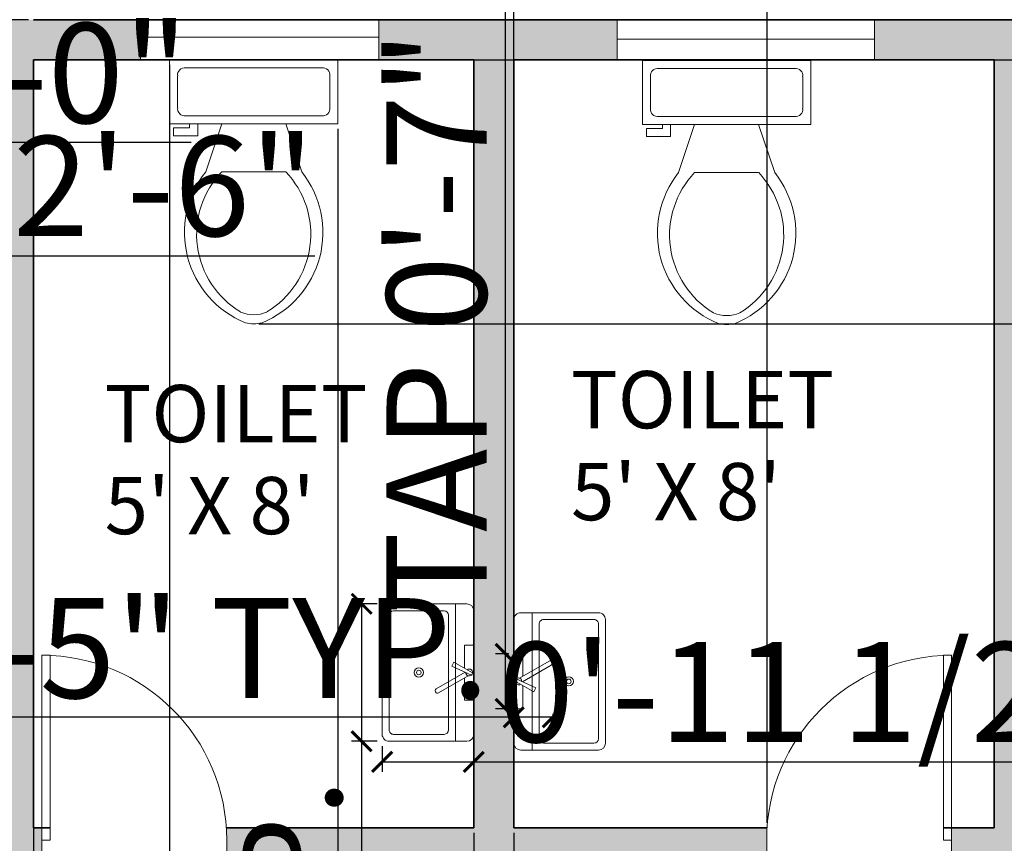
# Model space of a CAD drawing. Units: inches. Extents: x 1763 to 2368, y 1500 to 2097.
# Tile 11 of 24: x 1956 to 2079, y 1883 to 1986. Entities that reach past the tile are written whole.
import ezdxf

# ---------------------------------------------------------------- set-up
doc = ezdxf.new("R2010")
doc.units = ezdxf.units.IN
for name, color, linetype, lineweight in [('A-ANNO-DIMS', 2, 'Continuous', 18), ('A-AREA-IDEN', 7, 'Continuous', 18), ('A-DOOR', 4, 'Continuous', 18), ('A-FLOR-FIXT', 9, 'Continuous', 18), ('A-WALL', 7, 'Continuous', 35), ('A-WALL-PATT', 7, 'Continuous', 13), ('windows', 1, 'Continuous', 18)]:
    doc.layers.add(name, color=color, linetype=linetype, lineweight=lineweight)
doc.styles.get("Standard").update_dxf_attribs({"font": 'arial.ttf'})
doc.dimstyles.new('ISO-25', dxfattribs={"dimtxt": 12.5, "dimasz": 2.5, "dimexe": 1.25, "dimexo": 0.625, "dimtad": 1, "dimdec": 0, "dimlunit": 4, "dimtxsty": 'Standard', "dimblk": 'ARCHTICK', "dimcen": 2.5, "dimclrd": 3, "dimclrt": 4, "dimadec": 0, "dimazin": 0, "dimtfac": 1, "dimtdec": 0, "dimtmove": 0, "dimatfit": 3, "dimfxl": 1, "dimarcsym": 0})

# ---------------------------------------------------------------- blocks, each defined once
blk = doc.blocks.new('*U3')
for p, q in [((0, 0), (0, -6)), ((40, 0), (40, -6))]:
    blk.add_line(p, q)
blk.add_lwpolyline([(0, 0), (0, 40), (1.75, 40), (1.75, 0)], close=True)
blk.add_arc((0, 0), 40, 0, 90)
blk = doc.blocks.new('*U5')
for p, q in [((9.5, -6), (9.5, -2)), ((-10, -8.5), (-8, -8.5)), ((-10, -9.5), (-10, -8.5)), ((-8, -8.5), (-8, -8)), ((-7, -8), (-7, -9.5)), ((-4, -8), (-6, -14)), ((4, -8), (6, -14)), ((-7, -9.5), (-10, -9.5)), ((4, -14), (-4, -14))]:
    blk.add_line(p, q)
blk.add_lwpolyline([(10.5, -8), (10.5, 0), (-10.5, 0), (-10.5, -8)], close=True)
for points in [[(8.5, -1), (-8.5, -1)], [(-9.5, -2), (-9.5, -6)], [(-8.5, -7), (8.5, -7)]]:
    blk.add_lwpolyline(points)
for centre, radius, start, end in [((-8.62, -1.88), 0.884, 81.8699, 188.1301), ((8.62, -1.88), 0.884, 351.8699, 98.1301), ((-8.62, -6.12), 0.884, 171.8699, 278.1301), ((8.62, -6.12), 0.884, 261.8699, 8.1301), ((3.52, -21.58), 12.17, 141.4691, 247.9714), ((4.2, -21.82), 11.33, 136.3677, 238.9468), ((-3.52, -21.58), 12.17, 292.0284, 38.5307), ((-4.2, -21.82), 11.33, 301.053, 43.6321), ((0, -27.88), 4, 245.7318, 294.2682), ((0, -29), 4, 254.8605, 285.1395)]:
    blk.add_arc(centre, radius, start, end)
blk = doc.blocks.new('Faucet - single handle top')
for p, q in [((0.08, -0.26), (-2.26, -4.34)), ((-1.37, -4.79), (0.55, -0.5)), ((-0.06, -1.9), (3.57, -8.18)), ((4.43, -7.68), (0.72, -1.24)), ((-2.26, -4.34), (-1.37, -4.79))]:
    blk.add_line(p, q)
for points in [[(-0.92, -2), (-6, -2), (-6, 0), (6, 0), (6, -2), (1.16, -2)], [(-0.01, -2), (-0.12, -2)]]:
    blk.add_lwpolyline(points)
for centre, radius, start, end in [((0, -1), 0.75, 269.2246, 216.2304), ((4, -7.93), 0.5, 210, 30)]:
    blk.add_arc(centre, radius, start, end)
blk = doc.blocks.new('Sink-single - 30 in top')
blk.add_line((-15, -3.999996), (15, -3.999996))
for points in [[(-13.5, 0), (13.5, 0)], [(-15, -18.499996), (-15, -1.5)], [(15, -1.5), (15, -18.499996)], [(-12.5, -5.499996), (12.5, -5.499996)], [(-13.5, -17.499996), (-13.5, -6.499996)], [(13.5, -6.499996), (13.5, -17.499996)], [(12.5, -18.499996), (-12.5, -18.499996)], [(13.5, -19.999996), (-13.5, -19.999996)]]:
    blk.add_lwpolyline(points)
for radius in [1, 0.5]:
    blk.add_circle((0, -11.999996), radius)
for centre, radius, start, end in [((-13.5, -1.5), 1.5, 90, 180), ((13.5, -1.5), 1.5, 0, 90), ((-12.5, -6.499996), 1, 90, 180), ((12.5, -6.499996), 1, 0, 90), ((-13.5, -18.499996), 1.5, 180, 270), ((-12.5, -17.499996), 1, 180, 270), ((12.5, -17.499996), 1, 270, 0), ((13.5, -18.499996), 1.5, 270, 0)]:
    blk.add_arc(centre, radius, start, end)
blk = doc.blocks.new('_ArchTick')
at = {"color": 0, "linetype": 'ByBlock', "const_width": 0.15}
blk.add_lwpolyline([(-0.5, -0.5), (0.5, 0.5)], dxfattribs=at)
blk = doc.blocks.new('*D31')
at = {"layer": 'A-ANNO-DIMS', "color": 0, "lineweight": -2, "transparency": 16777216}
for p, q in [((1880.68, 1960.65), (1880.68, 1955.52)), ((1910.68, 1960.65), (1910.68, 1955.52))]:
    blk.add_line(p, q, dxfattribs=at)
at = {"layer": 'A-ANNO-DIMS', "color": 3, "lineweight": -2, "transparency": 16777216}
for p, q in [((1880.68, 1956.77), (1910.68, 1956.77)), ((1910.68, 1956.77), (1993.21, 1956.77))]:
    blk.add_line(p, q, dxfattribs=at)
at = {"layer": 'Defpoints', "color": 0, "transparency": 16777216}
for p in [(1880.68, 1961.27), (1910.68, 1961.27), (1910.68, 1956.77)]:
    blk.add_point(p, dxfattribs=at)
at = {"layer": 'A-ANNO-DIMS', "color": 3, "lineweight": -2, "transparency": 16777216, "xscale": 2.5, "yscale": 2.5, "zscale": 2.5, "rotation": 180}
blk.add_blockref('_ArchTick', (1880.68, 1956.77), dxfattribs=at)
at = {"layer": 'A-ANNO-DIMS', "color": 3, "lineweight": -2, "transparency": 16777216, "xscale": 2.5, "yscale": 2.5, "zscale": 2.5}
blk.add_blockref('_ArchTick', (1910.68, 1956.77), dxfattribs=at)
at = {"layer": 'A-ANNO-DIMS', "color": 4, "transparency": 16777216, "insert": (1953.2, 1963.86), "char_height": 12.5, "attachment_point": 5}
blk.add_mtext('SINK 2\'-6"', dxfattribs=at)
blk = doc.blocks.new('*D33')
at = {"layer": 'A-ANNO-DIMS', "color": 0, "lineweight": -2, "transparency": 16777216}
for p, q in [((2001.02, 1913.28), (1997.82, 1913.28)), ((2001.02, 1896.11), (1997.82, 1896.11))]:
    blk.add_line(p, q, dxfattribs=at)
at = {"layer": 'A-ANNO-DIMS', "color": 3, "lineweight": -2, "transparency": 16777216}
for p, q in [((1999.07, 1913.28), (1999.07, 1896.11)), ((1999.07, 1896.11), (1999.07, 1770.61))]:
    blk.add_line(p, q, dxfattribs=at)
at = {"layer": 'Defpoints', "color": 0, "transparency": 16777216}
for p in [(2001.64, 1913.28), (1999.07, 1896.11), (2001.64, 1896.11)]:
    blk.add_point(p, dxfattribs=at)
at = {"layer": 'A-ANNO-DIMS', "color": 3, "lineweight": -2, "transparency": 16777216, "xscale": 2.5, "yscale": 2.5, "zscale": 2.5}
for p, rotation in [((1999.07, 1913.28), 90), ((1999.07, 1896.11), 270)]:
    blk.add_blockref('_ArchTick', p, dxfattribs=dict(at, rotation=rotation))
at = {"layer": 'A-ANNO-DIMS', "color": 4, "transparency": 16777216, "insert": (1991.98, 1832.11), "char_height": 12.5, "attachment_point": 5, "rotation": 90}
blk.add_mtext('SINK 1\'-5" TYP.', dxfattribs=at)
blk = doc.blocks.new('*D34')
at = {"layer": 'A-ANNO-DIMS', "color": 0, "lineweight": -2, "transparency": 16777216}
for p, q in [((2001.64, 1895.48), (2001.64, 1892.28)), ((2013.09, 1895.48), (2013.09, 1892.28))]:
    blk.add_line(p, q, dxfattribs=at)
at = {"layer": 'A-ANNO-DIMS', "color": 3, "lineweight": -2, "transparency": 16777216}
for p, q in [((2001.64, 1893.53), (2013.09, 1893.53)), ((2013.09, 1893.53), (2131.87, 1893.53))]:
    blk.add_line(p, q, dxfattribs=at)
at = {"layer": 'Defpoints', "color": 0, "transparency": 16777216}
for p in [(2001.64, 1896.11), (2013.09, 1896.11), (2013.09, 1893.53)]:
    blk.add_point(p, dxfattribs=at)
at = {"layer": 'A-ANNO-DIMS', "color": 3, "lineweight": -2, "transparency": 16777216, "xscale": 2.5, "yscale": 2.5, "zscale": 2.5, "rotation": 180}
blk.add_blockref('_ArchTick', (2001.64, 1893.53), dxfattribs=at)
at = {"layer": 'A-ANNO-DIMS', "color": 3, "lineweight": -2, "transparency": 16777216, "xscale": 2.5, "yscale": 2.5, "zscale": 2.5}
blk.add_blockref('_ArchTick', (2013.09, 1893.53), dxfattribs=at)
at = {"layer": 'A-ANNO-DIMS', "color": 4, "transparency": 16777216, "insert": (2073.73, 1900.62), "char_height": 12.5, "attachment_point": 5}
blk.add_mtext('0\'-11 1/2" TYP.', dxfattribs=at)
blk = doc.blocks.new('*D35')
at = {"layer": 'A-ANNO-DIMS', "color": 0, "lineweight": -2, "transparency": 16777216}
for p, q in [((1889.68, 1972.15), (1889.68, 1969.72)), ((1901.68, 1972.15), (1901.68, 1969.72))]:
    blk.add_line(p, q, dxfattribs=at)
at = {"layer": 'A-ANNO-DIMS', "color": 3, "lineweight": -2, "transparency": 16777216}
for p, q in [((1889.68, 1970.97), (1901.68, 1970.97)), ((1901.68, 1970.97), (1977.79, 1970.97))]:
    blk.add_line(p, q, dxfattribs=at)
at = {"layer": 'Defpoints', "color": 0, "transparency": 16777216}
for p in [(1889.68, 1972.77), (1901.68, 1972.77), (1901.68, 1970.97)]:
    blk.add_point(p, dxfattribs=at)
at = {"layer": 'A-ANNO-DIMS', "color": 3, "lineweight": -2, "transparency": 16777216, "xscale": 2.5, "yscale": 2.5, "zscale": 2.5, "rotation": 180}
blk.add_blockref('_ArchTick', (1889.68, 1970.97), dxfattribs=at)
at = {"layer": 'A-ANNO-DIMS', "color": 3, "lineweight": -2, "transparency": 16777216, "xscale": 2.5, "yscale": 2.5, "zscale": 2.5}
blk.add_blockref('_ArchTick', (1901.68, 1970.97), dxfattribs=at)
at = {"layer": 'A-ANNO-DIMS', "color": 4, "transparency": 16777216, "insert": (1940.99, 1977.98), "char_height": 12.5, "attachment_point": 5}
blk.add_mtext('TAP 1\'-0"', dxfattribs=at)
blk = doc.blocks.new('*D37')
at = {"layer": 'A-ANNO-DIMS', "color": 3, "lineweight": -2, "transparency": 16777216}
for p, q in [((2017.06, 1907.01), (2017.06, 2026.09)), ((2017.06, 1900.14), (2017.06, 1907.01))]:
    blk.add_line(p, q, dxfattribs=at)
at = {"layer": 'A-ANNO-DIMS', "color": 0, "lineweight": -2, "transparency": 16777216}
for p, q in [((2017.47, 1907.01), (2015.81, 1907.01)), ((2017.47, 1900.14), (2015.81, 1900.14))]:
    blk.add_line(p, q, dxfattribs=at)
at = {"layer": 'Defpoints', "color": 0, "transparency": 16777216}
for p in [(2017.06, 1907.01), (2018.09, 1907.01), (2018.09, 1900.14)]:
    blk.add_point(p, dxfattribs=at)
at = {"layer": 'A-ANNO-DIMS', "color": 3, "lineweight": -2, "transparency": 16777216, "xscale": 2.5, "yscale": 2.5, "zscale": 2.5}
for p, rotation in [((2017.06, 1907.01), 90), ((2017.06, 1900.14), 270)]:
    blk.add_blockref('_ArchTick', p, dxfattribs=dict(at, rotation=rotation))
at = {"layer": 'A-ANNO-DIMS', "color": 4, "transparency": 16777216, "insert": (2010.05, 1967.8), "char_height": 12.5, "attachment_point": 5, "rotation": 90}
blk.add_mtext('TAP 0\'-7" TYP.', dxfattribs=at)
blk = doc.blocks.new('*D38')
at = {"layer": 'A-ANNO-DIMS', "color": 0, "lineweight": -2, "transparency": 16777216}
for p, q in [((2018.09, 1899.52), (2018.09, 1897.86)), ((2022.96, 1899.52), (2022.96, 1897.86))]:
    blk.add_line(p, q, dxfattribs=at)
at = {"layer": 'A-ANNO-DIMS', "color": 3, "lineweight": -2, "transparency": 16777216}
for p, q in [((2018.09, 1899.11), (1938.15, 1899.11)), ((2022.96, 1899.11), (2018.09, 1899.11))]:
    blk.add_line(p, q, dxfattribs=at)
at = {"layer": 'Defpoints', "color": 0, "transparency": 16777216}
for p in [(2018.09, 1900.14), (2022.96, 1900.14), (2018.09, 1899.11)]:
    blk.add_point(p, dxfattribs=at)
at = {"layer": 'A-ANNO-DIMS', "color": 3, "lineweight": -2, "transparency": 16777216, "xscale": 2.5, "yscale": 2.5, "zscale": 2.5, "rotation": 180}
blk.add_blockref('_ArchTick', (2018.09, 1899.11), dxfattribs=at)
at = {"layer": 'A-ANNO-DIMS', "color": 3, "lineweight": -2, "transparency": 16777216, "xscale": 2.5, "yscale": 2.5, "zscale": 2.5}
blk.add_blockref('_ArchTick', (2022.96, 1899.11), dxfattribs=at)
at = {"layer": 'A-ANNO-DIMS', "color": 4, "transparency": 16777216, "insert": (1976.87, 1906.12), "char_height": 12.5, "attachment_point": 5}
blk.add_mtext('0\'-5" TYP.', dxfattribs=at)
blk = doc.blocks.new('*D58')
at = {"layer": 'A-ANNO-DIMS', "color": 0, "lineweight": -2, "transparency": 16777216}
for p, q in [((1871.68, 1635.9), (1871.68, 2072.02)), ((1927.07, 1635.9), (1927.07, 2072.02))]:
    blk.add_line(p, q, dxfattribs=at)
at = {"layer": 'A-ANNO-DIMS', "color": 3, "lineweight": -2, "transparency": 16777216}
for p, q in [((1871.68, 2070.77), (1927.07, 2070.77)), ((1927.07, 2070.77), (1993.68, 2070.77))]:
    blk.add_line(p, q, dxfattribs=at)
at = {"layer": 'Defpoints', "color": 0, "transparency": 16777216}
for p in [(1927.07, 2070.77), (1871.68, 1635.27), (1927.07, 1635.27)]:
    blk.add_point(p, dxfattribs=at)
at = {"layer": 'A-ANNO-DIMS', "color": 3, "lineweight": -2, "transparency": 16777216, "xscale": 2.5, "yscale": 2.5, "zscale": 2.5, "rotation": 180}
blk.add_blockref('_ArchTick', (1871.68, 2070.77), dxfattribs=at)
at = {"layer": 'A-ANNO-DIMS', "color": 3, "lineweight": -2, "transparency": 16777216, "xscale": 2.5, "yscale": 2.5, "zscale": 2.5}
blk.add_blockref('_ArchTick', (1927.07, 2070.77), dxfattribs=at)
at = {"layer": 'A-ANNO-DIMS', "color": 4, "transparency": 16777216, "insert": (1961.63, 2077.86), "char_height": 12.5, "attachment_point": 5}
blk.add_mtext('4\'-7 1/2"', dxfattribs=at)
blk = doc.blocks.new('*D72')
at = {"layer": 'A-ANNO-DIMS', "color": 0, "lineweight": -2, "transparency": 16777216}
for p, q in [((2018.09, 1885.9), (2018.09, 2072.02)), ((2049.74, 1885.9), (2049.74, 2072.02))]:
    blk.add_line(p, q, dxfattribs=at)
at = {"layer": 'A-ANNO-DIMS', "color": 3, "lineweight": -2, "transparency": 16777216}
for p, q in [((2018.09, 2070.77), (2049.74, 2070.77)), ((2049.74, 2070.77), (2116.06, 2070.77))]:
    blk.add_line(p, q, dxfattribs=at)
at = {"layer": 'Defpoints', "color": 0, "transparency": 16777216}
for p in [(2049.74, 2070.77), (2018.09, 1885.27), (2049.74, 1885.27)]:
    blk.add_point(p, dxfattribs=at)
at = {"layer": 'A-ANNO-DIMS', "color": 3, "lineweight": -2, "transparency": 16777216, "xscale": 2.5, "yscale": 2.5, "zscale": 2.5, "rotation": 180}
blk.add_blockref('_ArchTick', (2018.09, 2070.77), dxfattribs=at)
at = {"layer": 'A-ANNO-DIMS', "color": 3, "lineweight": -2, "transparency": 16777216, "xscale": 2.5, "yscale": 2.5, "zscale": 2.5}
blk.add_blockref('_ArchTick', (2049.74, 2070.77), dxfattribs=at)
at = {"layer": 'A-ANNO-DIMS', "color": 4, "transparency": 16777216, "insert": (2084.15, 2077.86), "char_height": 12.5, "attachment_point": 5}
blk.add_mtext('2\'-7 1/2"', dxfattribs=at)
blk = doc.blocks.new('*D77')
at = {"layer": 'A-ANNO-DIMS', "color": 0, "lineweight": -2, "transparency": 16777216}
for p, q in [((1975.09, 1972.65), (1975.09, 1509.91)), ((1996.09, 1972.65), (1996.09, 1509.91))]:
    blk.add_line(p, q, dxfattribs=at)
at = {"layer": 'A-ANNO-DIMS', "color": 3, "lineweight": -2, "transparency": 16777216}
for p, q in [((1975.09, 1511.16), (1996.09, 1511.16)), ((1996.09, 1511.16), (2031.89, 1511.16))]:
    blk.add_line(p, q, dxfattribs=at)
at = {"layer": 'Defpoints', "color": 0, "transparency": 16777216}
for p in [(1975.09, 1973.27), (1996.09, 1973.27), (1996.09, 1511.16)]:
    blk.add_point(p, dxfattribs=at)
at = {"layer": 'A-ANNO-DIMS', "color": 3, "lineweight": -2, "transparency": 16777216, "xscale": 2.5, "yscale": 2.5, "zscale": 2.5, "rotation": 180}
blk.add_blockref('_ArchTick', (1975.09, 1511.16), dxfattribs=at)
at = {"layer": 'A-ANNO-DIMS', "color": 3, "lineweight": -2, "transparency": 16777216, "xscale": 2.5, "yscale": 2.5, "zscale": 2.5}
blk.add_blockref('_ArchTick', (1996.09, 1511.16), dxfattribs=at)
at = {"layer": 'A-ANNO-DIMS', "color": 4, "transparency": 16777216, "insert": (2015.24, 1518.16), "char_height": 12.5, "attachment_point": 5}
blk.add_mtext('1\'-9"', dxfattribs=at)
blk = doc.blocks.new('*D78')
at = {"layer": 'A-ANNO-DIMS', "color": 0, "lineweight": -2, "transparency": 16777216}
for p, q in [((1996.72, 1981.27), (2217.84, 1981.27)), ((1986.22, 1948.27), (2217.84, 1948.27))]:
    blk.add_line(p, q, dxfattribs=at)
at = {"layer": 'A-ANNO-DIMS', "color": 3, "lineweight": -2, "transparency": 16777216}
for p, q in [((2216.59, 1981.27), (2216.59, 1948.27)), ((2216.59, 1948.27), (2216.59, 1911.08))]:
    blk.add_line(p, q, dxfattribs=at)
at = {"layer": 'Defpoints', "color": 0, "transparency": 16777216}
for p in [(1996.09, 1981.27), (1985.59, 1948.27), (2216.59, 1948.27)]:
    blk.add_point(p, dxfattribs=at)
at = {"layer": 'A-ANNO-DIMS', "color": 3, "lineweight": -2, "transparency": 16777216, "xscale": 2.5, "yscale": 2.5, "zscale": 2.5}
for p, rotation in [((2216.59, 1981.27), 90), ((2216.59, 1948.27), 270)]:
    blk.add_blockref('_ArchTick', p, dxfattribs=dict(at, rotation=rotation))
at = {"layer": 'A-ANNO-DIMS', "color": 4, "transparency": 16777216, "insert": (2209.58, 1928.43), "char_height": 12.5, "attachment_point": 5, "rotation": 90}
blk.add_mtext('2\'-9"', dxfattribs=at)
blk = doc.blocks.new('*D81')
at = {"layer": 'A-ANNO-DIMS', "color": 3, "lineweight": -2, "transparency": 16777216}
for p, q in [((1788.85, 1866.87), (1788.85, 1912.38)), ((1788.85, 1843.77), (1788.85, 1866.87))]:
    blk.add_line(p, q, dxfattribs=at)
at = {"layer": 'A-ANNO-DIMS', "color": 0, "lineweight": -2, "transparency": 16777216}
for p, q in [((2077.47, 1866.87), (1787.6, 1866.87)), ((2077.47, 1843.77), (1787.6, 1843.77))]:
    blk.add_line(p, q, dxfattribs=at)
at = {"layer": 'Defpoints', "color": 0, "transparency": 16777216}
for p in [(1788.85, 1866.87), (2078.09, 1866.87), (2078.09, 1843.77)]:
    blk.add_point(p, dxfattribs=at)
at = {"layer": 'A-ANNO-DIMS', "color": 3, "lineweight": -2, "transparency": 16777216, "xscale": 2.5, "yscale": 2.5, "zscale": 2.5}
for p, rotation in [((1788.85, 1866.87), 90), ((1788.85, 1843.77), 270)]:
    blk.add_blockref('_ArchTick', p, dxfattribs=dict(at, rotation=rotation))
at = {"layer": 'A-ANNO-DIMS', "color": 4, "transparency": 16777216, "insert": (1781.95, 1890.87), "char_height": 12.5, "attachment_point": 5, "rotation": 90}
blk.add_mtext('1\'-11"', dxfattribs=at)
blk = doc.blocks.new('*D82')
at = {"layer": 'A-ANNO-DIMS', "color": 3, "lineweight": -2, "transparency": 16777216}
for p, q in [((1788.85, 1843.77), (1788.85, 1909.87)), ((1788.85, 1837.27), (1788.85, 1843.77))]:
    blk.add_line(p, q, dxfattribs=at)
at = {"layer": 'A-ANNO-DIMS', "color": 0, "lineweight": -2, "transparency": 16777216}
for p, q in [((2077.47, 1843.77), (1787.6, 1843.77)), ((2077.47, 1837.27), (1787.6, 1837.27))]:
    blk.add_line(p, q, dxfattribs=at)
at = {"layer": 'Defpoints', "color": 0, "transparency": 16777216}
for p in [(1788.85, 1843.77), (2078.09, 1843.77), (2078.09, 1837.27)]:
    blk.add_point(p, dxfattribs=at)
at = {"layer": 'A-ANNO-DIMS', "color": 3, "lineweight": -2, "transparency": 16777216, "xscale": 2.5, "yscale": 2.5, "zscale": 2.5}
for p, rotation in [((1788.85, 1843.77), 90), ((1788.85, 1837.27), 270)]:
    blk.add_blockref('_ArchTick', p, dxfattribs=dict(at, rotation=rotation))
at = {"layer": 'A-ANNO-DIMS', "color": 4, "transparency": 16777216, "insert": (1781.77, 1878.07), "char_height": 12.5, "attachment_point": 5, "rotation": 90}
blk.add_mtext('0\'-6 1/2"', dxfattribs=at)
blk = doc.blocks.new('*D85')
at = {"layer": 'A-ANNO-DIMS', "color": 0, "lineweight": -2, "transparency": 16777216}
for p, q in [((1957.47, 1986.27), (1787.6, 1986.27)), ((1958.51, 1880.27), (1787.6, 1880.27))]:
    blk.add_line(p, q, dxfattribs=at)
at = {"layer": 'A-ANNO-DIMS', "color": 3, "lineweight": -2, "transparency": 16777216}
blk.add_line((1788.85, 1986.27), (1788.85, 1880.27), dxfattribs=at)
at = {"layer": 'Defpoints', "color": 0, "transparency": 16777216}
for p in [(1958.09, 1986.27), (1788.85, 1880.27), (1959.13, 1880.27)]:
    blk.add_point(p, dxfattribs=at)
at = {"layer": 'A-ANNO-DIMS', "color": 3, "lineweight": -2, "transparency": 16777216, "xscale": 2.5, "yscale": 2.5, "zscale": 2.5}
for p, rotation in [((1788.85, 1986.27), 90), ((1788.85, 1880.27), 270)]:
    blk.add_blockref('_ArchTick', p, dxfattribs=dict(at, rotation=rotation))
at = {"layer": 'A-ANNO-DIMS', "color": 4, "transparency": 16777216, "insert": (1781.85, 1933.27), "char_height": 12.5, "attachment_point": 5, "rotation": 90}
blk.add_mtext('8\'-10"', dxfattribs=at)
blk = doc.blocks.new('*D86')
at = {"layer": 'A-ANNO-DIMS', "color": 0, "lineweight": -2, "transparency": 16777216}
for p, q in [((2013.09, 1884.65), (2013.09, 1509.91)), ((2018.09, 1884.65), (2018.09, 1509.91))]:
    blk.add_line(p, q, dxfattribs=at)
at = {"layer": 'A-ANNO-DIMS', "color": 3, "lineweight": -2, "transparency": 16777216}
for p, q in [((2013.09, 1511.16), (2018.09, 1511.16)), ((2018.09, 1511.16), (2055.07, 1511.16))]:
    blk.add_line(p, q, dxfattribs=at)
at = {"layer": 'Defpoints', "color": 0, "transparency": 16777216}
for p in [(2013.09, 1885.27), (2018.09, 1885.27), (2018.09, 1511.16)]:
    blk.add_point(p, dxfattribs=at)
at = {"layer": 'A-ANNO-DIMS', "color": 3, "lineweight": -2, "transparency": 16777216, "xscale": 2.5, "yscale": 2.5, "zscale": 2.5, "rotation": 180}
blk.add_blockref('_ArchTick', (2013.09, 1511.16), dxfattribs=at)
at = {"layer": 'A-ANNO-DIMS', "color": 3, "lineweight": -2, "transparency": 16777216, "xscale": 2.5, "yscale": 2.5, "zscale": 2.5}
blk.add_blockref('_ArchTick', (2018.09, 1511.16), dxfattribs=at)
at = {"layer": 'A-ANNO-DIMS', "color": 4, "transparency": 16777216, "insert": (2037.83, 1518.16), "char_height": 12.5, "attachment_point": 5}
blk.add_mtext('0\'-5"', dxfattribs=at)
blk = doc.blocks.new('*D87')
at = {"layer": 'A-ANNO-DIMS', "color": 0, "lineweight": -2, "transparency": 16777216}
for p, q in [((1958.09, 1980.65), (1958.09, 1509.91)), ((1975.09, 1980.65), (1975.09, 1509.91))]:
    blk.add_line(p, q, dxfattribs=at)
at = {"layer": 'A-ANNO-DIMS', "color": 3, "lineweight": -2, "transparency": 16777216}
for p, q in [((1958.09, 1511.16), (1975.09, 1511.16)), ((1975.09, 1511.16), (2010.89, 1511.16))]:
    blk.add_line(p, q, dxfattribs=at)
at = {"layer": 'Defpoints', "color": 0, "transparency": 16777216}
for p in [(1958.09, 1981.27), (1975.09, 1981.27), (1975.09, 1511.16)]:
    blk.add_point(p, dxfattribs=at)
at = {"layer": 'A-ANNO-DIMS', "color": 3, "lineweight": -2, "transparency": 16777216, "xscale": 2.5, "yscale": 2.5, "zscale": 2.5, "rotation": 180}
blk.add_blockref('_ArchTick', (1958.09, 1511.16), dxfattribs=at)
at = {"layer": 'A-ANNO-DIMS', "color": 3, "lineweight": -2, "transparency": 16777216, "xscale": 2.5, "yscale": 2.5, "zscale": 2.5}
blk.add_blockref('_ArchTick', (1975.09, 1511.16), dxfattribs=at)
at = {"layer": 'A-ANNO-DIMS', "color": 4, "transparency": 16777216, "insert": (1994.24, 1518.16), "char_height": 12.5, "attachment_point": 5}
blk.add_mtext('1\'-5"', dxfattribs=at)

msp = doc.modelspace()

# ---------------------------------------------------------------- hatches: boundary and pattern name
at = {"layer": 'A-WALL-PATT'}
h = msp.add_hatch(color=256, dxfattribs=at)
h.dxf.hatch_style = 1
h.paths.add_polyline_path([(1838.09, 2034.27), (1838.09, 2043.27), (1829.09, 2043.27), (1829.09, 1953.39), (1838.09, 1953.39)])
h.paths.add_polyline_path([(1838.09, 1913.1), (1829.09, 1913.1), (1829.09, 1862.2), (1838.09, 1862.2)])
h.paths.add_polyline_path([(1838.09, 1825.59), (1829.09, 1825.59), (1829.09, 1738.64), (1838.09, 1738.64)])
h.paths.add_polyline_path([(1895.59, 1885.27), (1838.09, 1885.27), (1838.09, 1880.27), (1895.59, 1880.27)])
h.paths.add_polyline_path([(1857.39, 1784.27), (1838.09, 1784.27), (1838.09, 1779.27), (1857.39, 1779.27)])
h.paths.add_polyline_path([(1958.09, 1981.27), (1971.46, 1981.27), (1971.46, 1986.27), (1968.57, 1986.27), (1958.09, 1986.27), (1953.09, 1986.27), (1927.39, 1986.27), (1927.39, 1981.27), (1953.09, 1981.27), (1953.09, 1885.27), (1932.01, 1885.27), (1932.01, 1880.27), (1959.13, 1880.27), (1959.13, 1883.74), (1959.13, 1885.27), (1958.09, 1885.27)])
h.paths.add_polyline_path([(2018.09, 1981.27), (2031.02, 1981.27), (2031.02, 1986.27), (2018.09, 1986.27), (2013.09, 1986.27), (2001.23, 1986.27), (2001.23, 1981.27), (2013.09, 1981.27), (2013.09, 1885.27), (1982.18, 1885.27, -0.016629), (1982.23, 1883.74), (1982.23, 1880.27), (2049.69, 1880.27), (2049.69, 1883.74, -0.016629), (2049.74, 1885.27), (2018.09, 1885.27)])
h.paths.add_polyline_path([(2083.09, 1981.27), (2120.61, 1981.27), (2120.61, 1986.27), (2083.09, 1986.27), (2078.09, 1986.27), (2063.14, 1986.27), (2063.14, 1981.27), (2078.09, 1981.27), (2078.09, 1885.27), (2072.78, 1885.27), (2072.78, 1883.74), (2072.78, 1880.27), (2078.09, 1880.27), (2078.09, 1866.87), (2081.56, 1866.87, -0.016629), (2083.09, 1866.82)])
h.paths.add_polyline_path([(1871.68, 1635.27), (1838.09, 1635.27), (1838.09, 1626.27), (1871.68, 1626.27)], flags=17)
h.paths.add_polyline_path([(2100.58, 1688.27), (2060.09, 1688.27), (2060.09, 1679.27), (2100.58, 1679.27)], flags=17)
h.paths.add_polyline_path([(2180.09, 1688.27), (2148.74, 1688.27), (2148.74, 1679.27), (2180.09, 1679.27)], flags=17)
h.paths.add_polyline_path([(2189.09, 1746.22), (2180.09, 1746.22), (2180.09, 1743.42), (2180.12, 1743.42), (2180.12, 1726.72), (2180.09, 1572.27), (2034.91, 1572.27), (2034.91, 1565.6), (2034.91, 1563.27), (2189.09, 1563.27)])
h.paths.add_polyline_path([(2060.09, 1802.35, -0.016629), (2058.56, 1802.3), (2055.09, 1802.3), (2055.09, 1635.27), (2042.48, 1635.27), (2042.48, 1629.74), (2042.48, 1626.27), (2055.09, 1626.27), (2055.09, 1599.27), (2040.27, 1599.27), (2040.27, 1590.27), (2060.09, 1590.27)])
h.paths.add_polyline_path([(2019.39, 1629.74, -0.060569), (2020.06, 1635.27), (1995.09, 1635.27), (1990.09, 1635.27), (1927.07, 1635.27), (1927.07, 1626.27), (1990.09, 1626.27), (1990.09, 1590.27), (1995.09, 1590.27), (2005.2, 1590.27), (2005.2, 1599.27), (1995.09, 1599.27), (1995.09, 1626.27), (2019.39, 1626.27)])
edge = h.paths.add_edge_path()
edge.add_line((2180.09, 1837.27), (2167.2, 1837.27))
edge.add_spline(control_points=[(2167.2, 1837.27), (2167.19, 1837.27), (2167.18, 1837.27), (2167.18, 1837.27)], knot_values=[168.955493, 168.955493, 168.955493, 168.955493, 169.065871, 169.065871, 169.065871, 169.065871], degree=3, periodic=0)
edge.add_spline(control_points=[(2167.18, 1837.27), (2166.56, 1837.38), (2166.33, 1846.16), (2165.71, 1846.24)], knot_values=[159.864705, 159.864705, 159.864705, 159.864705, 168.955493, 168.955493, 168.955493, 168.955493], degree=3, periodic=0)
edge.add_line((2167.12, 1837.27), (2163.16, 1837.27))
edge.add_spline(control_points=[(2163.16, 1837.27), (2163.16, 1837.27), (2163.16, 1837.27), (2163.15, 1837.27)], knot_values=[150.537172, 150.537172, 150.537172, 150.537172, 150.553797, 150.553797, 150.553797, 150.553797], degree=3, periodic=0)
edge.add_spline(control_points=[(2163.15, 1837.27), (2162.29, 1837.29), (2161.59, 1846.23), (2160.88, 1846.24)], knot_values=[141.293426, 141.293426, 141.293426, 141.293426, 150.537172, 150.537172, 150.537172, 150.537172], degree=3, periodic=0)
edge.add_line((2163.08, 1837.27), (2158.7, 1837.27))
edge.add_spline(control_points=[(2158.7, 1837.27), (2158.7, 1837.27), (2158.7, 1837.27), (2158.7, 1837.27)], knot_values=[132.033544, 132.033544, 132.033544, 132.033544, 132.049151, 132.049151, 132.049151, 132.049151], degree=3, periodic=0)
edge.add_spline(control_points=[(2158.7, 1837.27), (2157.97, 1837.29), (2157.26, 1846.23), (2156.39, 1846.24)], knot_values=[122.786021, 122.786021, 122.786021, 122.786021, 132.033544, 132.033544, 132.033544, 132.033544], degree=3, periodic=0)
edge.add_line((2158.63, 1837.27), (2153.84, 1837.27))
edge.add_spline(control_points=[(2153.84, 1837.27), (2153.83, 1837.27), (2153.82, 1837.27), (2153.82, 1837.27)], knot_values=[113.451585, 113.451585, 113.451585, 113.451585, 113.562103, 113.562103, 113.562103, 113.562103], degree=3, periodic=0)
edge.add_spline(control_points=[(2153.82, 1837.27), (2153.17, 1837.38), (2152.88, 1846.19), (2152.4, 1846.24)], knot_values=[0, 0, 0, 0, 9.081854, 9.081854, 9.081854, 9.081854], degree=3, periodic=0)
edge.add_line((2153.76, 1837.27), (2150.39, 1837.27))
edge.add_spline(control_points=[(2150.39, 1837.27), (2150.38, 1837.27), (2150.37, 1837.27), (2150.36, 1837.27)], knot_values=[95.069382, 95.069382, 95.069382, 95.069382, 95.17519, 95.17519, 95.17519, 95.17519], degree=3, periodic=0)
edge.add_spline(control_points=[(2150.36, 1837.27), (2149.49, 1837.37), (2148.42, 1846.19), (2147.59, 1846.24)], knot_values=[85.824599, 85.824599, 85.824599, 85.824599, 95.069382, 95.069382, 95.069382, 95.069382], degree=3, periodic=0)
edge.add_line((2150.29, 1837.27), (2145.43, 1837.27))
edge.add_spline(control_points=[(2145.43, 1837.27), (2145.43, 1837.27), (2145.42, 1837.27), (2145.42, 1837.27)], knot_values=[76.505559, 76.505559, 76.505559, 76.505559, 76.547811, 76.547811, 76.547811, 76.547811], degree=3, periodic=0)
edge.add_spline(control_points=[(2145.42, 1837.27), (2144.68, 1837.31), (2143.8, 1846.19), (2142.95, 1846.24)], knot_values=[67.23945, 67.23945, 67.23945, 67.23945, 76.505559, 76.505559, 76.505559, 76.505559], degree=3, periodic=0)
edge.add_line((2145.35, 1837.27), (2134.57, 1837.27))
edge.add_spline(control_points=[(2134.57, 1837.27), (2134.57, 1837.27), (2134.56, 1837.27), (2134.56, 1837.27)], knot_values=[39.001463, 39.001463, 39.001463, 39.001463, 39.045107, 39.045107, 39.045107, 39.045107], degree=3, periodic=0)
edge.add_spline(control_points=[(2134.56, 1837.27), (2133.87, 1837.31), (2133.4, 1845.85), (2132.33, 1846.24)], knot_values=[29.79778, 29.79778, 29.79778, 29.79778, 39.001463, 39.001463, 39.001463, 39.001463], degree=3, periodic=0)
edge.add_line((2134.5, 1837.27), (2128.08, 1837.27))
edge.add_spline(control_points=[(2128.08, 1837.27), (2128.03, 1837.26), (2127.98, 1837.26), (2127.93, 1837.27)], knot_values=[19.482067, 19.482067, 19.482067, 19.482067, 19.869396, 19.869396, 19.869396, 19.869396], degree=3, periodic=0)
edge.add_spline(control_points=[(2125.01, 1846.24), (2126.16, 1844.66), (2126.82, 1837.57), (2127.93, 1837.27)], knot_values=[10.389805, 10.389805, 10.389805, 10.389805, 19.482067, 19.482067, 19.482067, 19.482067], degree=3, periodic=0)
edge.add_line((2127.93, 1837.27), (2083.09, 1837.27))
edge.add_line((2083.09, 1837.27), (2083.09, 1843.77))
edge.add_line((2083.09, 1843.77), (2081.56, 1843.77))
edge.add_line((2081.56, 1843.77), (2078.09, 1843.77))
edge.add_line((2078.09, 1843.77), (2078.09, 1837.27))
edge.add_line((2078.09, 1837.27), (2055.09, 1837.27))
edge.add_line((2055.09, 1837.27), (2055.09, 1825.4))
edge.add_line((2055.09, 1825.4), (2058.56, 1825.4))
edge.add_line((2058.56, 1825.4), (2060.09, 1825.4))
edge.add_line((2060.09, 1825.4), (2060.09, 1832.27))
edge.add_line((2060.09, 1832.27), (2122.44, 1832.27))
edge.add_spline(control_points=[(2122.44, 1832.27), (2122.73, 1832.58), (2123.01, 1832.62), (2123.28, 1832.27)], knot_values=[5.972033, 5.972033, 5.972033, 5.972033, 8.057258, 8.057258, 8.057258, 8.057258], degree=3, periodic=0)
edge.add_line((2123.28, 1832.27), (2137.95, 1832.27))
edge.add_spline(control_points=[(2137.95, 1832.27), (2137.96, 1832.27), (2137.97, 1832.27), (2137.98, 1832.27)], knot_values=[53.926862, 53.926862, 53.926862, 53.926862, 54.030075, 54.030075, 54.030075, 54.030075], degree=3, periodic=0)
edge.add_spline(control_points=[(2139.72, 1825.02), (2139.28, 1825.06), (2138.67, 1832.18), (2137.98, 1832.27)], knot_values=[54.030075, 54.030075, 54.030075, 54.030075, 61.445194, 61.445194, 61.445194, 61.445194], degree=3, periodic=0)
edge.add_line((2138.05, 1832.27), (2140.96, 1832.27))
edge.add_spline(control_points=[(2140.96, 1832.27), (2140.97, 1832.27), (2140.98, 1832.27), (2140.99, 1832.27)], knot_values=[68.854182, 68.854182, 68.854182, 68.854182, 68.971237, 68.971237, 68.971237, 68.971237], degree=3, periodic=0)
edge.add_spline(control_points=[(2143.19, 1825.02), (2142.44, 1825.07), (2141.56, 1832.16), (2140.99, 1832.27)], knot_values=[68.971237, 68.971237, 68.971237, 68.971237, 76.444911, 76.444911, 76.444911, 76.444911], degree=3, periodic=0)
edge.add_line((2141.04, 1832.27), (2145.43, 1832.27))
edge.add_spline(control_points=[(2145.43, 1832.27), (2145.44, 1832.27), (2145.45, 1832.27), (2145.46, 1832.27)], knot_values=[84.039047, 84.039047, 84.039047, 84.039047, 84.124041, 84.124041, 84.124041, 84.124041], degree=3, periodic=0)
edge.add_spline(control_points=[(2148.11, 1825.02), (2147.34, 1825.02), (2146.3, 1832.19), (2145.46, 1832.27)], knot_values=[84.124041, 84.124041, 84.124041, 84.124041, 91.773891, 91.773891, 91.773891, 91.773891], degree=3, periodic=0)
edge.add_line((2145.54, 1832.27), (2150.39, 1832.27))
edge.add_spline(control_points=[(2150.39, 1832.27), (2150.42, 1832.28), (2150.45, 1832.28), (2150.47, 1832.27)], knot_values=[99.381577, 99.381577, 99.381577, 99.381577, 99.573457, 99.573457, 99.573457, 99.573457], degree=3, periodic=0)
edge.add_spline(control_points=[(2153.97, 1825.02), (2153.09, 1825.28), (2151.53, 1832.1), (2150.47, 1832.27)], knot_values=[99.573457, 99.573457, 99.573457, 99.573457, 107.218357, 107.218357, 107.218357, 107.218357], degree=3, periodic=0)
edge.add_line((2150.57, 1832.27), (2155.6, 1832.27))
edge.add_spline(control_points=[(2155.6, 1832.27), (2155.6, 1832.27), (2155.61, 1832.27), (2155.62, 1832.27)], knot_values=[114.933058, 114.933058, 114.933058, 114.933058, 115.013624, 115.013624, 115.013624, 115.013624], degree=3, periodic=0)
edge.add_spline(control_points=[(2158.28, 1825.02), (2157.4, 1825.07), (2156.25, 1832.2), (2155.62, 1832.27)], knot_values=[115.013624, 115.013624, 115.013624, 115.013624, 122.616269, 122.616269, 122.616269, 122.616269], degree=3, periodic=0)
edge.add_line((2155.68, 1832.27), (2165.19, 1832.27))
edge.add_spline(control_points=[(2165.19, 1832.27), (2165.2, 1832.27), (2165.2, 1832.27), (2165.2, 1832.27)], knot_values=[145.488477, 145.488477, 145.488477, 145.488477, 145.516379, 145.516379, 145.516379, 145.516379], degree=3, periodic=0)
edge.add_spline(control_points=[(2167.45, 1825.02), (2166.96, 1825.02), (2166.06, 1832.25), (2165.2, 1832.27)], knot_values=[145.516379, 145.516379, 145.516379, 145.516379, 153.105469, 153.105469, 153.105469, 153.105469], degree=3, periodic=0)
edge.add_line((2165.29, 1832.27), (2168.93, 1832.27))
edge.add_spline(control_points=[(2168.93, 1832.27), (2168.98, 1832.29), (2169.04, 1832.29), (2169.1, 1832.27)], knot_values=[160.517439, 160.517439, 160.517439, 160.517439, 160.939723, 160.939723, 160.939723, 160.939723], degree=3, periodic=0)
edge.add_spline(control_points=[(2171.09, 1828.64), (2170.35, 1830.37), (2169.62, 1832.09), (2169.1, 1832.27)], knot_values=[160.939723, 160.939723, 160.939723, 160.939723, 164.738835, 164.738835, 164.738835, 164.738835], degree=3, periodic=0)
edge.add_line((2169.1, 1832.27), (2180.09, 1832.27))
edge.add_line((2180.09, 1832.27), (2180.09, 1837.27))
h.paths.add_polyline_path([(2189.09, 1885.52), (2180.09, 1885.52), (2180.09, 1813.32), (2180.12, 1813.32), (2180.12, 1796.62), (2180.12, 1795.26), (2189.09, 1795.26)])
h.paths.add_polyline_path([(2180.09, 1986.27), (2166.28, 1986.27), (2166.28, 1981.27), (2180.09, 1981.27)])
h.paths.add_polyline_path([(2189.09, 2043.27), (2180.09, 2043.27), (2180.09, 2034.27), (2180.09, 1934.11), (2189.09, 1934.11)])
h.paths.add_polyline_path([(1838.09, 1681.59), (1829.09, 1681.59), (1829.09, 1563.27), (2003.86, 1563.27), (2003.86, 1565.6), (2003.86, 1572.27), (1838.09, 1572.27)])

# ---------------------------------------------------------------- linework, layer by layer
at = {"layer": 'A-WALL'}
for p, q in [((1958.09, 1986.27), (2013.09, 1986.27)), ((2018.09, 1986.27), (2013.09, 1986.27)), ((2018.09, 1986.27), (2078.09, 1986.27)), ((2083.09, 1986.27), (2078.09, 1986.27)), ((1958.09, 1885.27), (1958.09, 1981.27)), ((1958.09, 1981.27), (2013.09, 1981.27)), ((2013.09, 1885.27), (2013.09, 1981.27)), ((2018.09, 1885.27), (2018.09, 1981.27)), ((2018.09, 1981.27), (2078.09, 1981.27)), ((2078.09, 1885.27), (2078.09, 1981.27)), ((1958.09, 1885.27), (1960.14, 1885.27)), ((1982.18, 1885.27), (2013.09, 1885.27)), ((2018.09, 1885.27), (2049.74, 1885.27)), ((2071.77, 1885.27), (2078.09, 1885.27))]:
    msp.add_line(p, q, dxfattribs=at)
at = {"layer": 'windows'}
for p, q in [((2001.23, 1986.27), (1968.57, 1986.27)), ((1971.46, 1986.27), (1971.46, 1981.27)), ((2001.23, 1981.27), (2001.23, 1986.27)), ((2031.02, 1986.27), (2031.02, 1981.27)), ((2063.14, 1986.27), (2031.02, 1986.27)), ((2063.14, 1981.27), (2063.14, 1986.27)), ((1971.46, 1984.07), (2001.23, 1984.07)), ((2031.02, 1983.82), (2063.14, 1983.82)), ((1971.46, 1981.27), (2001.23, 1981.27)), ((2031.02, 1981.27), (2063.14, 1981.27))]:
    msp.add_line(p, q, dxfattribs=at)

# ---------------------------------------------------------------- block references
at = {"layer": 'A-DOOR', "yscale": 0.5774759422388936, "zscale": 0.5774759422388936}
for p, xscale in [((1959.13, 1883.74), 0.5774759422388936), ((2072.78, 1883.74), -0.5774759422388936)]:
    msp.add_blockref('*U3', p, dxfattribs=dict(at, xscale=xscale))
at = {"layer": 'A-FLOR-FIXT'}
for p in [(1985.59, 1981.27), (2044.68, 1981.17)]:
    msp.add_blockref('*U5', p, dxfattribs=at)
at = {"layer": 'A-FLOR-FIXT', "xscale": 0.5723750491206686, "yscale": 0.5723750491206686, "zscale": 0.5723750491206686}
for name, p, rotation in [('Sink-single - 30 in top', (2013.09, 1904.69), 270), ('Sink-single - 30 in top', (2018.09, 1903.58), 89.99999999999999), ('Faucet - single handle top', (2013.09, 1904.69), 270), ('Faucet - single handle top', (2018.09, 1903.58), 89.99999999999999)]:
    msp.add_blockref(name, p, dxfattribs=dict(at, rotation=rotation))

# ---------------------------------------------------------------- texts
at = {"layer": 'A-AREA-IDEN'}
for s, p in [('TOILET', (2025.24, 1935.21)), ('TOILET', (1966.97, 1933.47)), ("5' X 8'", (2025.24, 1923.72)), ("5' X 8'", (1966.97, 1921.98))]:
    msp.add_text(s, height=7.155, dxfattribs=at).set_placement(p)

# ---------------------------------------------------------------- dimensions: what is measured, and where the dimension line sits
at = {"layer": 'A-ANNO-DIMS'}
for base, p1, p2, picture, middle in [((1927.07, 2070.77), (1871.68, 1635.27), (1927.07, 1635.27), '*D58', (1961.63, 2077.86)), ((2049.7368, 2070.7727), (2018.0918, 1885.2727), (2049.7368, 1885.2727), '*D72', (2084.1459, 2077.8609)), ((1975.09, 1511.16), (1958.09, 1981.27), (1975.09, 1981.27), '*D87', (1994.24, 1518.16)), ((1996.09, 1511.16), (1975.09, 1973.27), (1996.09, 1973.27), '*D77', (2015.24, 1518.16)), ((2018.09, 1511.16), (2013.09, 1885.27), (2018.09, 1885.27), '*D86', (2037.83, 1518.16))]:
    dim = msp.add_linear_dim(base=base, p1=p1, p2=p2, dimstyle='ISO-25', override={"dimdec": 1, "dimlfac": 1, "dimrnd": 0, "dimzin": 1, "dimdsep": 46, "dimlunit": 4, "dimfrac": 2}, dxfattribs=at)
    dim.commit()
    dim.dimension.update_dxf_attribs({"geometry": picture, "text_midpoint": middle})
for base, p1, p2, angle, text, picture, middle in [((2017.06, 1907.01), (2018.09, 1900.14), (2018.09, 1907.01), 90, 'TAP <> TYP.', '*D37', (2010.05, 1967.8)), ((2018.09, 1899.11), (2022.96, 1900.14), (2018.09, 1900.14), 180, '<> TYP.', '*D38', (1976.87, 1906.12)), ((1999.07, 1896.11), (2001.64, 1913.28), (2001.64, 1896.11), 270, 'SINK <> TYP.', '*D33', (1991.98, 1832.11))]:
    dim = msp.add_linear_dim(base=base, p1=p1, p2=p2, angle=angle, text=text, dimstyle='ISO-25', override={"dimdec": 1, "dimlfac": 1, "dimrnd": 0, "dimzin": 1, "dimdsep": 46, "dimlunit": 4, "dimfrac": 2}, dxfattribs=at)
    dim.commit()
    dim.dimension.update_dxf_attribs({"geometry": picture, "text_midpoint": middle})
for base, p1, p2, text, picture, middle in [((1901.68, 1970.97), (1889.68, 1972.77), (1901.68, 1972.77), 'TAP <>', '*D35', (1940.99, 1977.98)), ((1910.68, 1956.77), (1880.68, 1961.27), (1910.68, 1961.27), 'SINK <>', '*D31', (1953.2, 1963.86)), ((2013.0918, 1893.5307), (2001.6443, 1896.1064), (2013.0918, 1896.1064), '<> TYP.', '*D34', (2073.733, 1900.6189))]:
    dim = msp.add_linear_dim(base=base, p1=p1, p2=p2, text=text, dimstyle='ISO-25', override={"dimdec": 1, "dimlfac": 1, "dimrnd": 0, "dimzin": 1, "dimdsep": 46, "dimlunit": 4, "dimfrac": 2}, dxfattribs=at)
    dim.commit()
    dim.dimension.update_dxf_attribs({"geometry": picture, "text_midpoint": middle})
for base, p1, p2, picture, middle in [((1788.85, 1880.27), (1958.09, 1986.27), (1959.13, 1880.27), '*D85', (1781.85, 1933.27)), ((2216.59, 1948.27), (1996.09, 1981.27), (1985.59, 1948.27), '*D78', (2209.58, 1928.43)), ((1788.85, 1866.87), (2078.09, 1843.77), (2078.09, 1866.87), '*D81', (1781.95, 1890.87)), ((1788.85, 1843.77), (2078.09, 1837.27), (2078.09, 1843.77), '*D82', (1781.77, 1878.07))]:
    dim = msp.add_linear_dim(base=base, p1=p1, p2=p2, angle=90, dimstyle='ISO-25', override={"dimdec": 1, "dimlfac": 1, "dimrnd": 0, "dimzin": 1, "dimdsep": 46, "dimlunit": 4, "dimfrac": 2}, dxfattribs=at)
    dim.commit()
    dim.dimension.update_dxf_attribs({"geometry": picture, "text_midpoint": middle})

doc.saveas('drawing.dxf')
